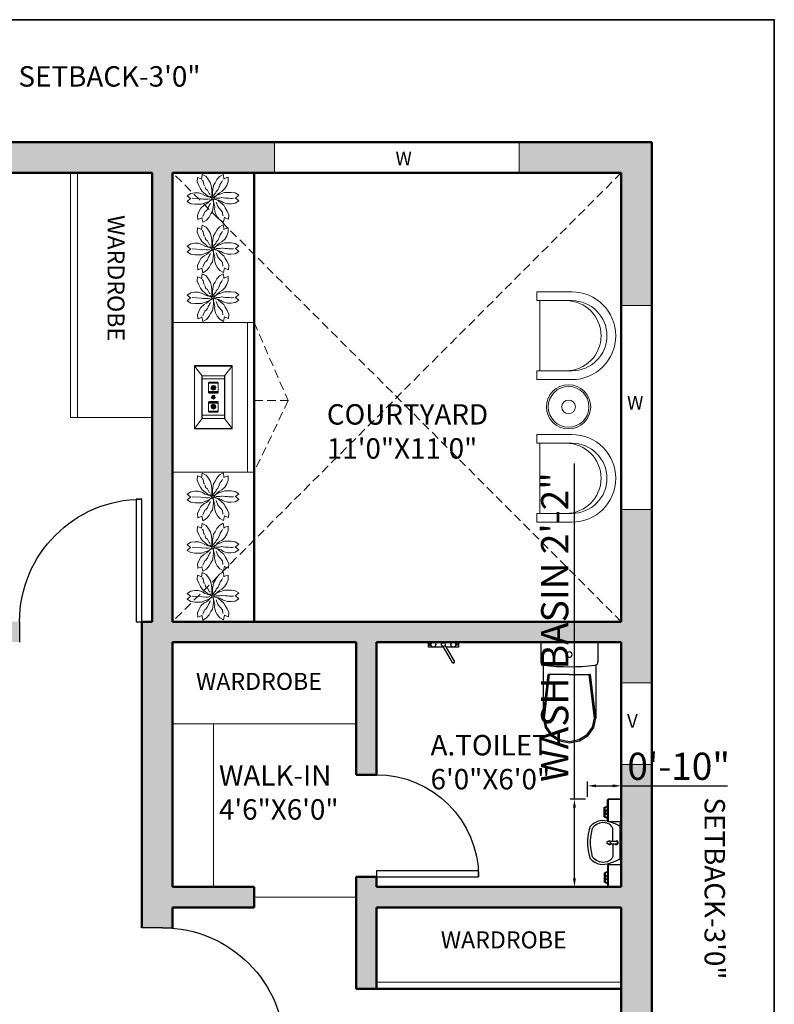
# Model space of a CAD drawing. Units: inches. Extents: x 3354 to 4308, y 1668 to 2317.
# Tile 11 of 11: x 4033 to 4255, y 2005 to 2294. Entities that reach past the tile are written whole.
import ezdxf

# ---------------------------------------------------------------- set-up
doc = ezdxf.new("R2010")
doc.units = ezdxf.units.IN
doc.linetypes.add('DASHED', pattern=[19.05, 12.7, -6.35])
for name, color, linetype, lineweight in [('A-ANNO-DIMS', 2, 'Continuous', 18), ('A-ANNO-TEXT', 7, 'Continuous', 18), ('A-AREA-IDEN', 3, 'Continuous', 18), ('A-DOOR', 3, 'Continuous', 25), ('A-FLOR-FIXT', 8, 'Continuous', 18), ('A-FLOR-OVHD', 8, 'DASHED', 18), ('A-FURN', 8, 'Continuous', 18), ('A-GLAZ', 4, 'Continuous', 18), ('A-WALL', 7, 'Continuous', 50), ('A-WALL-PATT', 8, 'Continuous', 13), ('C-PROP', 1, 'Continuous', 35), ('L-PLNT', 84, 'Continuous', 13)]:
    doc.layers.add(name, color=color, linetype=linetype, lineweight=lineweight)
doc.layers.add('SANTEH', color=7, linetype='Continuous')
doc.styles.get("Standard").update_dxf_attribs({"font": 'arial.ttf'})
doc.dimstyles.new('ISO-25', dxfattribs={"dimtxt": 8, "dimasz": 2.5, "dimexe": 1.25, "dimexo": 0.625, "dimtad": 1, "dimdec": 1, "dimlunit": 3, "dimtxsty": 'Standard', "dimcen": 2.5, "dimadec": 0, "dimazin": 0, "dimtfac": 1, "dimtdec": 1, "dimtmove": 0, "dimatfit": 3, "dimfxl": 1, "dimarcsym": 0})

# ---------------------------------------------------------------- blocks, each defined once
blk = doc.blocks.new('12PSTG07')
at = {"color": 0, "linetype": 'ByBlock'}
for p, q in [((0, 15), (-12, 15)), ((0, 12), (0, 15)), ((-12, 12), (0, 12)), ((-1, -12), (-1, 12)), ((-12, -12), (0, -12)), ((0, -12), (0, -15)), ((0, -15), (-12, -15))]:
    blk.add_line(p, q, dxfattribs=at)
for centre, radius in [((-12, 0), 15), ((-12, 0), 12), ((-10, 0), 12)]:
    blk.add_arc(centre, radius, 90, 270, dxfattribs=at)
blk = doc.blocks.new('*U3')
for p, q in [((0, 0), (0, -6)), ((36, 0), (36, -6))]:
    blk.add_line(p, q)
blk.add_lwpolyline([(0, 0), (0, 36), (1.75, 36), (1.75, 0)], close=True)
blk.add_arc((0, 0), 36, 0, 90)
blk = doc.blocks.new('ml')
for p, q in [((3455.3311, 1925.7742), (3455.3307, 1925.7627)), ((3455.3431, 1925.7698), (3455.3311, 1925.7742)), ((3455.3419, 1925.7691), (3455.3441, 1925.7817)), ((3455.3441, 1925.7817), (3455.3543, 1925.7763)), ((3455.3543, 1925.7763), (3455.3608, 1925.7679)), ((3455.3892, 1925.7768), (3455.3826, 1925.7684)), ((3455.3993, 1925.7823), (3455.3892, 1925.7768)), ((3455.4016, 1925.7697), (3455.3993, 1925.7823)), ((3455.4003, 1925.7704), (3455.4124, 1925.7747)), ((3455.4124, 1925.7747), (3455.4127, 1925.7632)), ((3455.3307, 1925.7627), (3455.3347, 1925.7528)), ((3455.3347, 1925.7528), (3455.3396, 1925.7443)), ((3455.3435, 1925.7672), (3455.3464, 1925.7643)), ((3455.3464, 1925.7643), (3455.3485, 1925.7554)), ((3455.3485, 1925.7554), (3455.3499, 1925.7524)), ((3455.3514, 1925.7499), (3455.3528, 1925.744)), ((3455.3608, 1925.7679), (3455.3657, 1925.7594)), ((3455.3657, 1925.7594), (3455.368, 1925.7482)), ((3455.368, 1925.7482), (3455.3679, 1925.7458)), ((3455.3688, 1925.7419), (3455.3679, 1925.7458)), ((3455.3721, 1925.7432), (3455.3738, 1925.7534)), ((3455.3738, 1925.7534), (3455.3777, 1925.76)), ((3455.3826, 1925.7684), (3455.3777, 1925.76)), ((3455.3855, 1925.743), (3455.3866, 1925.7454)), ((3455.3866, 1925.7454), (3455.3873, 1925.7469)), ((3455.3873, 1925.7469), (3455.3888, 1925.7494)), ((3455.3888, 1925.7494), (3455.3895, 1925.7504)), ((3455.3895, 1925.7504), (3455.3912, 1925.7564)), ((3455.3912, 1925.7564), (3455.3927, 1925.7588)), ((3455.3927, 1925.7588), (3455.3938, 1925.7598)), ((3455.3938, 1925.7598), (3455.3952, 1925.7623)), ((3455.3952, 1925.7623), (3455.3977, 1925.7658)), ((3455.4038, 1925.7449), (3455.3952, 1925.7373)), ((3455.4087, 1925.7534), (3455.4038, 1925.7449)), ((3455.4127, 1925.7632), (3455.4087, 1925.7534)), ((3455.304, 1925.7261), (3455.3138, 1925.7322)), ((3455.3138, 1925.7178), (3455.304, 1925.7261)), ((3455.3138, 1925.7193), (3455.304, 1925.711)), ((3455.3138, 1925.7322), (3455.3243, 1925.7337)), ((3455.317, 1925.7192), (3455.341, 1925.7177)), ((3455.3243, 1925.7337), (3455.3341, 1925.7337)), ((3455.3341, 1925.7337), (3455.345, 1925.73)), ((3455.3434, 1925.7376), (3455.3396, 1925.7443)), ((3455.3514, 1925.7311), (3455.3434, 1925.7376)), ((3455.345, 1925.73), (3455.3509, 1925.7263)), ((3455.3509, 1925.7263), (3455.3573, 1925.7241)), ((3455.3579, 1925.7256), (3455.3514, 1925.7311)), ((3455.3528, 1925.744), (3455.3579, 1925.7405)), ((3455.3573, 1925.7241), (3455.3659, 1925.7219)), ((3455.3579, 1925.7405), (3455.3622, 1925.7316)), ((3455.3656, 1925.7214), (3455.3579, 1925.7256)), ((3455.3622, 1925.7316), (3455.3639, 1925.7301)), ((3455.3639, 1925.7301), (3455.3647, 1925.7291)), ((3455.3643, 1925.7251), (3455.3672, 1925.7211)), ((3455.3707, 1925.7212), (3455.3656, 1925.7214)), ((3455.3659, 1925.7219), (3455.3697, 1925.7189)), ((3455.3697, 1925.7189), (3455.367, 1925.7145)), ((3455.3688, 1925.7216), (3455.3688, 1925.7419)), ((3455.3691, 1925.7345), (3455.3715, 1925.726)), ((3455.3707, 1925.7348), (3455.3721, 1925.7432)), ((3455.3708, 1925.726), (3455.3707, 1925.7348)), ((3455.3715, 1925.726), (3455.3707, 1925.7212)), ((3455.3733, 1925.7215), (3455.3708, 1925.726)), ((3455.3778, 1925.7232), (3455.3733, 1925.7215)), ((3455.3736, 1925.7261), (3455.3765, 1925.7301)), ((3455.3748, 1925.7194), (3455.3775, 1925.7238)), ((3455.3785, 1925.7164), (3455.3748, 1925.7194)), ((3455.3765, 1925.7301), (3455.3776, 1925.7316)), ((3455.3775, 1925.7238), (3455.385, 1925.7283)), ((3455.3776, 1925.7316), (3455.3794, 1925.7335)), ((3455.384, 1925.7296), (3455.3778, 1925.7232)), ((3455.3794, 1925.7335), (3455.3805, 1925.737)), ((3455.3798, 1925.7196), (3455.383, 1925.7196)), ((3455.3805, 1925.737), (3455.3826, 1925.739)), ((3455.3826, 1925.739), (3455.3848, 1925.7414)), ((3455.383, 1925.7196), (3455.3905, 1925.7196)), ((3455.3891, 1925.734), (3455.384, 1925.7296)), ((3455.3848, 1925.7414), (3455.3855, 1925.743)), ((3455.385, 1925.7283), (3455.393, 1925.7312)), ((3455.3952, 1925.7373), (3455.3891, 1925.734)), ((3455.3905, 1925.7196), (3455.3945, 1925.7211)), ((3455.393, 1925.7312), (3455.4026, 1925.7349)), ((3455.3945, 1925.7211), (3455.397, 1925.7211)), ((3455.3995, 1925.7206), (3455.4045, 1925.7196)), ((3455.4026, 1925.7349), (3455.4103, 1925.7348)), ((3455.4045, 1925.7196), (3455.4103, 1925.7196)), ((3455.4201, 1925.7348), (3455.4103, 1925.7348)), ((3455.4103, 1925.7196), (3455.4139, 1925.7192)), ((3455.4139, 1925.7192), (3455.4189, 1925.7187)), ((3455.4189, 1925.7187), (3455.4225, 1925.7187)), ((3455.4306, 1925.7333), (3455.4201, 1925.7348)), ((3455.4225, 1925.7187), (3455.426, 1925.7192)), ((3455.4404, 1925.7273), (3455.4306, 1925.7333)), ((3455.4306, 1925.719), (3455.4404, 1925.7273)), ((3455.4306, 1925.7205), (3455.4404, 1925.7122)), ((3455.304, 1925.711), (3455.3138, 1925.705)), ((3455.3138, 1925.705), (3455.3243, 1925.7035)), ((3455.3243, 1925.7035), (3455.3341, 1925.7035)), ((3455.3418, 1925.7034), (3455.3341, 1925.7035)), ((3455.3357, 1925.6849), (3455.3406, 1925.6934)), ((3455.3406, 1925.6934), (3455.3492, 1925.701)), ((3455.341, 1925.7177), (3455.3453, 1925.7167)), ((3455.3514, 1925.7071), (3455.3418, 1925.7034)), ((3455.3453, 1925.7167), (3455.3489, 1925.7172)), ((3455.3489, 1925.7172), (3455.3543, 1925.7167)), ((3455.3492, 1925.701), (3455.3553, 1925.7043)), ((3455.3595, 1925.71), (3455.3514, 1925.7071)), ((3455.3543, 1925.7167), (3455.3597, 1925.7167)), ((3455.3553, 1925.7043), (3455.3605, 1925.7088)), ((3455.3582, 1925.6924), (3455.3597, 1925.6949)), ((3455.367, 1925.7145), (3455.3595, 1925.71)), ((3455.3597, 1925.7167), (3455.3636, 1925.7177)), ((3455.3597, 1925.6949), (3455.3608, 1925.6974)), ((3455.3605, 1925.7088), (3455.3667, 1925.7151)), ((3455.3608, 1925.6974), (3455.3618, 1925.6993)), ((3455.3618, 1925.6993), (3455.3632, 1925.7023)), ((3455.3632, 1925.7023), (3455.3647, 1925.7048)), ((3455.3647, 1925.7048), (3455.3661, 1925.7067)), ((3455.3667, 1925.7151), (3455.3712, 1925.7168)), ((3455.3723, 1925.6951), (3455.3706, 1925.6849)), ((3455.3712, 1925.7168), (3455.3736, 1925.7123)), ((3455.3738, 1925.7035), (3455.3723, 1925.6951)), ((3455.373, 1925.7123), (3455.3737, 1925.7171)), ((3455.3753, 1925.7038), (3455.373, 1925.7123)), ((3455.3736, 1925.7123), (3455.3738, 1925.7035)), ((3455.3737, 1925.7171), (3455.3789, 1925.7169)), ((3455.3767, 1925.6971), (3455.3753, 1925.7038)), ((3455.3764, 1925.6901), (3455.3767, 1925.6971)), ((3455.3871, 1925.7142), (3455.3785, 1925.7164)), ((3455.3789, 1925.7169), (3455.3865, 1925.7127)), ((3455.3804, 1925.7089), (3455.385, 1925.6972)), ((3455.385, 1925.6972), (3455.3976, 1925.683)), ((3455.3865, 1925.7127), (3455.3931, 1925.7072)), ((3455.3935, 1925.712), (3455.3871, 1925.7142)), ((3455.3931, 1925.7072), (3455.4011, 1925.7007)), ((3455.3994, 1925.7083), (3455.3935, 1925.712)), ((3455.4103, 1925.7046), (3455.3994, 1925.7083)), ((3455.4011, 1925.7007), (3455.4048, 1925.694)), ((3455.4097, 1925.6855), (3455.4048, 1925.694)), ((3455.4201, 1925.7046), (3455.4103, 1925.7046)), ((3455.4306, 1925.7061), (3455.4201, 1925.7046)), ((3455.4404, 1925.7122), (3455.4306, 1925.7061)), ((3455.3317, 1925.6751), (3455.3357, 1925.6849)), ((3455.3321, 1925.6636), (3455.3317, 1925.6751)), ((3455.3441, 1925.6679), (3455.3321, 1925.6636)), ((3455.3429, 1925.6686), (3455.3451, 1925.656)), ((3455.3457, 1925.6716), (3455.3504, 1925.6835)), ((3455.3504, 1925.6835), (3455.3532, 1925.6849)), ((3455.3532, 1925.6849), (3455.355, 1925.6874)), ((3455.355, 1925.6874), (3455.3575, 1925.6904)), ((3455.3553, 1925.6615), (3455.3618, 1925.6699)), ((3455.3575, 1925.6904), (3455.3582, 1925.6924)), ((3455.3618, 1925.6699), (3455.3667, 1925.6783)), ((3455.3706, 1925.6849), (3455.3667, 1925.6783)), ((3455.3787, 1925.6789), (3455.3764, 1925.6901)), ((3455.3836, 1925.6704), (3455.3787, 1925.6789)), ((3455.3902, 1925.662), (3455.3836, 1925.6704)), ((3455.3976, 1925.683), (3455.3985, 1925.6734)), ((3455.4026, 1925.6692), (3455.4003, 1925.6566)), ((3455.4013, 1925.6685), (3455.4134, 1925.6641)), ((3455.4137, 1925.6756), (3455.4097, 1925.6855)), ((3455.4134, 1925.6641), (3455.4137, 1925.6756)), ((3455.3451, 1925.656), (3455.3553, 1925.6615)), ((3455.4003, 1925.6566), (3455.3902, 1925.662))]:
    blk.add_line(p, q)
blk = doc.blocks.new('12PLMP48')
for p, q in [((-4.94, 8.22), (-5, 8.31)), ((-5, 8.31), (5, 8.31)), ((-5, -8.31), (-5, 8.31)), ((-2.96, 5.62), (-4.94, 8.22)), ((4.94, 8.22), (-4.94, 8.22)), ((-4.94, 8.22), (-4.94, -8.22)), ((2.96, 5.62), (4.94, 8.22)), ((5, 8.31), (4.94, 8.22)), ((4.94, 8.22), (4.94, -8.22)), ((5, 8.31), (5, -8.31)), ((-2.94, 5.59), (-3, 5.62)), ((-3, 5.62), (3, 5.62)), ((-3, -5.63), (-3, 5.62)), ((2.94, 5.59), (-2.94, 5.59)), ((-2.94, 5.59), (-2.94, -5.59)), ((3, 5.62), (2.94, 5.59)), ((2.94, -5.59), (2.94, 5.59)), ((3, -5.63), (3, 5.62)), ((2.94, 4.81), (-2.94, 4.81)), ((-1.13, 3.94), (-1.25, 3.81)), ((-1.13, 3.84), (-1.25, 3.72)), ((-1.25, 3.81), (-1.25, 1.22)), ((-1.25, 3.72), (1.25, 3.72)), ((1.13, 3.94), (-1.13, 3.94)), ((-1.13, 3.84), (-1.13, 3.94)), ((1.13, 3.84), (-1.13, 3.84)), ((-0.62, 2.61), (-0.4, 2.98)), ((0, 2.5), (-0.62, 2.61)), ((-0.54, 2.19), (-0.62, 2.61)), ((-0.32, 2.88), (-0.49, 2.59)), ((-0.43, 2.58), (-0.28, 2.83)), ((0, 3.12), (-0.4, 2.98)), ((-0.4, 2.98), (-0.32, 2.88)), ((0, 3), (-0.32, 2.88)), ((-0.32, 2.88), (-0.32, 2.88)), ((-0.32, 2.88), (-0.28, 2.83)), ((-0.28, 2.83), (0, 2.94)), ((-0.28, 2.83), (0, 2.5)), ((-0.08, 2.6), (-0.12, 2.52)), ((0, 2.62), (-0.08, 2.6)), ((0, 2.5), (0, 3.12)), ((0, 3.12), (0.4, 2.98)), ((0.32, 2.88), (0, 3)), ((0, 2.94), (0.28, 2.83)), ((0, 2.5), (0.32, 2.88)), ((0.08, 2.6), (0, 2.62)), ((0.62, 2.61), (0, 2.5)), ((0.12, 2.52), (0.08, 2.6)), ((0.28, 2.83), (0.43, 2.58)), ((0.32, 2.88), (0.4, 2.98)), ((0.49, 2.59), (0.32, 2.88)), ((0.32, 2.88), (0.32, 2.88)), ((0.4, 2.98), (0.62, 2.61)), ((0.54, 2.19), (0.62, 2.61)), ((1.25, 3.81), (1.13, 3.94)), ((1.13, 3.84), (1.13, 3.94)), ((1.25, 3.72), (1.13, 3.84)), ((1.25, 1.22), (1.25, 3.81)), ((-1.13, 1.41), (-1.25, 1.53)), ((-1.25, 1.53), (1.25, 1.53)), ((-1.13, 1.25), (-1.25, 1.37)), ((-1.25, 1.22), (-1.13, 1.09)), ((1.13, 1.41), (-1.13, 1.41)), ((-1.13, 1.41), (-1.13, 1.09)), ((-1.13, 1.25), (1.13, 1.25)), ((-1.13, 1.09), (1.13, 1.09)), ((-0.38, 2.28), (-0.54, 2.19)), ((-0.54, 2.19), (-0.21, 1.91)), ((-0.49, 2.59), (-0.43, 2.25)), ((-0.49, -0.09), (-0.43, 0.25)), ((-0.38, 2.28), (-0.43, 2.58)), ((-0.43, 2.25), (-0.17, 2.03)), ((-0.43, 0.25), (-0.17, 0.47)), ((0, 2.5), (-0.38, 2.28)), ((-0.15, 2.09), (-0.38, 2.28)), ((-0.22, 0.12), (-0.25, -0.04)), ((-0.09, 0.23), (-0.22, 0.12)), ((-0.21, 1.91), (0, 2.5)), ((0.21, 1.91), (-0.21, 1.91)), ((-0.17, 2.03), (0.17, 2.03)), ((0.17, 0.47), (-0.17, 0.47)), ((0.15, 2.09), (-0.15, 2.09)), ((-0.12, 2.52), (-0.11, 2.44)), ((-0.12, -0.12), (-0.12, 0.12)), ((-0.12, 0.12), (0.12, 0.12)), ((-0.11, 2.44), (-0.04, 2.38)), ((-0.09, 0.23), (0.09, 0.23)), ((-0.04, 2.38), (0.04, 2.38)), ((0.54, 2.19), (0, 2.5)), ((0, 2.5), (0.21, 1.91)), ((0.04, 2.38), (0.11, 2.44)), ((0.22, 0.12), (0.09, 0.23)), ((0.11, 2.44), (0.12, 2.52)), ((0.12, 0.12), (0.12, -0.12)), ((0.38, 2.28), (0.15, 2.09)), ((0.17, 2.03), (0.43, 2.25)), ((0.43, 0.25), (0.17, 0.47)), ((0.21, 1.91), (0.54, 2.19)), ((0.25, -0.04), (0.22, 0.12)), ((0.43, 2.58), (0.38, 2.28)), ((0.43, 2.25), (0.49, 2.59)), ((0.43, 0.25), (0.49, -0.09)), ((1.25, 1.53), (1.13, 1.41)), ((1.13, 1.09), (1.13, 1.41)), ((1.13, 1.25), (1.25, 1.37)), ((1.13, 1.09), (1.25, 1.22)), ((-1.25, -1.22), (-1.13, -1.09)), ((-1.25, -1.22), (-1.25, -3.81)), ((-1.13, -1.25), (-1.25, -1.38)), ((-1.13, -1.41), (-1.25, -1.53)), ((-1.25, -1.53), (1.25, -1.53)), ((-1.13, -1.41), (-1.13, -1.09)), ((-1.13, -1.09), (1.13, -1.09)), ((1.13, -1.25), (-1.13, -1.25)), ((1.13, -1.41), (-1.13, -1.41)), ((-0.54, -2.19), (-0.62, -2.61)), ((0, -2.5), (-0.62, -2.61)), ((-0.21, -1.91), (-0.54, -2.19)), ((-0.54, -2.19), (0, -2.5)), ((-0.32, -0.38), (-0.49, -0.09)), ((-0.49, -2.59), (-0.43, -2.25)), ((-0.32, -2.88), (-0.49, -2.59)), ((-0.43, -2.25), (-0.17, -2.03)), ((-0.43, -2.58), (-0.38, -2.28)), ((-0.28, -2.84), (-0.43, -2.58)), ((-0.38, -2.28), (-0.15, -2.09)), ((-0.32, -0.38), (0, -0.5)), ((-0.16, -0.19), (-0.25, -0.04)), ((0.21, -1.91), (-0.21, -1.91)), ((0, -2.5), (-0.21, -1.91)), ((-0.17, -2.03), (0.17, -2.03)), ((0, -0.25), (-0.16, -0.19)), ((-0.15, -2.09), (0.15, -2.09)), ((0.12, -0.12), (-0.12, -0.12)), ((-0.11, -2.44), (-0.12, -2.52)), ((-0.12, -2.52), (-0.08, -2.6)), ((-0.04, -2.38), (-0.11, -2.44)), ((-0.08, -2.6), (0, -2.5)), ((0.04, -2.38), (-0.04, -2.38)), ((0.16, -0.19), (0, -0.25)), ((0.32, -0.38), (0, -0.5)), ((0, -2.5), (0.21, -1.91)), ((0.11, -2.44), (0, -2.5)), ((0, -3.13), (0, -2.5)), ((0, -2.5), (0.4, -2.98)), ((0.62, -2.61), (0, -2.5)), ((0.11, -2.44), (0.04, -2.38)), ((0.08, -2.6), (0.12, -2.52)), ((0.38, -2.28), (0.11, -2.44)), ((0.12, -2.52), (0.11, -2.44)), ((0.15, -2.09), (0.38, -2.28)), ((0.16, -0.19), (0.25, -0.04)), ((0.17, -2.03), (0.43, -2.25)), ((0.21, -1.91), (0.54, -2.19)), ((0.43, -2.58), (0.28, -2.84)), ((0.32, -0.38), (0.49, -0.09)), ((0.49, -2.59), (0.32, -2.88)), ((0.54, -2.19), (0.38, -2.28)), ((0.38, -2.28), (0.43, -2.58)), ((0.43, -2.25), (0.49, -2.59)), ((0.62, -2.61), (0.54, -2.19)), ((1.13, -1.41), (1.13, -1.09)), ((1.13, -1.09), (1.25, -1.22)), ((1.25, -1.38), (1.13, -1.25)), ((1.25, -1.53), (1.13, -1.41)), ((1.25, -3.81), (1.25, -1.22)), ((2.94, -4.69), (-2.94, -4.69)), ((-1.13, -3.84), (-1.25, -3.72)), ((-1.25, -3.72), (1.25, -3.72)), ((-1.25, -3.81), (-1.13, -3.94)), ((-1.13, -3.94), (-1.13, -3.84)), ((1.13, -3.84), (-1.13, -3.84)), ((-1.13, -3.94), (1.13, -3.94)), ((-0.62, -2.61), (-0.4, -2.98)), ((-0.4, -2.98), (-0.32, -2.88)), ((-0.4, -2.98), (0, -3.13)), ((-0.32, -2.88), (-0.28, -2.84)), ((0, -3), (-0.32, -2.88)), ((-0.28, -2.84), (-0.08, -2.6)), ((0, -2.94), (-0.28, -2.84)), ((-0.08, -2.6), (0, -2.63)), ((0, -2.63), (0.08, -2.6)), ((0.28, -2.84), (0, -2.94)), ((0.32, -2.88), (0, -3)), ((0, -3.13), (0.4, -2.98)), ((0.4, -2.98), (0.62, -2.61)), ((1.25, -3.72), (1.13, -3.84)), ((1.13, -3.94), (1.25, -3.81)), ((1.13, -3.94), (1.13, -3.84)), ((-4.94, -8.22), (-2.96, -5.63)), ((-2.94, -5.59), (-3, -5.63)), ((-3, -5.63), (3, -5.63)), ((-2.94, -5.59), (2.94, -5.59)), ((3, -5.63), (2.94, -5.59)), ((2.96, -5.63), (4.94, -8.22)), ((-4.94, -8.22), (-5, -8.31)), ((5, -8.31), (-5, -8.31)), ((4.94, -8.22), (-4.94, -8.22)), ((4.94, -8.22), (5, -8.31))]:
    blk.add_line(p, q)
blk = doc.blocks.new('*U2')
for p, q in [((0, 0), (0, -6)), ((30, 0), (30, -6))]:
    blk.add_line(p, q)
blk.add_lwpolyline([(0, 0), (0, 30), (1.75, 30), (1.75, 0)], close=True)
blk.add_arc((0, 0), 30, 0, 90)
blk = doc.blocks.new('WC 2 Symb_109')
at = {"layer": 'SANTEH'}
for p, q in [((0, 0), (0, 380)), ((0, 380), (132.4, 380)), ((153.6, 364.9), (506.8, 364.9)), ((506.3, 364.9), (215.7, 330.9)), ((506.3, 356), (215.7, 322)), ((215.7, 190), (215.7, 330.9)), ((215.7, 190), (215.7, 49.1)), ((153.8, 15.1), (506.8, 15.1)), ((506.3, 24), (215.7, 58)), ((506.3, 15.1), (215.7, 49.1)), ((0, 0), (132.4, 0))]:
    blk.add_line(p, q, dxfattribs=at)
for points in [[(154.6, 360.1), (153.9, 364.1), (152.3, 367.9), (150.2, 371.3), (147.4, 374.3), (144.1, 376.7), (140.5, 378.5), (136.5, 379.6), (132.4, 380)], [(154.6, 19.7), (158.6, 62.1), (161.4, 104.7), (163.1, 147.3), (163.7, 189.9), (163.1, 232.5), (161.4, 275.1), (158.6, 317.7), (154.6, 360.1)], [(506.3, 24), (565.5, 36.6), (615.7, 72.6), (649.2, 126.5), (661, 190), (649.2, 253.5), (615.7, 307.4), (565.5, 343.4), (506.3, 356)], [(506.8, 15.1), (569.2, 28.4), (622.2, 66.3), (657.6, 123.1), (670, 190), (657.6, 256.9), (622.2, 313.7), (569.2, 351.6), (506.8, 364.9)], [(132.4, 0), (136.5, 0.4), (140.4, 1.5), (144.1, 3.2), (147.3, 5.6), (150.1, 8.6), (152.3, 12), (153.8, 15.7), (154.6, 19.7)]]:
    blk.add_lwpolyline(points, dxfattribs=at)
blk.add_lwpolyline([(83.6, 208.5), (70.4, 203.1), (64.9, 190), (70.4, 176.9), (83.6, 171.5), (96.8, 176.9), (102.2, 190), (96.8, 203.1)], close=True, dxfattribs=at)
blk = doc.blocks.new('Faucet - kit sink top')
at = {"layer": 'SANTEH'}
for p, q in [((-5.5, -0.75), (-5.5, -1.25)), ((-4.94278, -0.75), (-5.5, -0.75)), ((-5.5, -1.25), (-4.94278, -1.25)), ((-0.14775, -1.7441), (3.56698, -8.1782)), ((4.43301, -7.6782), (0.71828, -1.2441)), ((4.94278, -0.75), (5.5, -0.75)), ((5.5, -1.25), (4.94278, -1.25)), ((5.5, -0.75), (5.5, -1.25))]:
    blk.add_line(p, q, dxfattribs=at)
blk.add_lwpolyline([(-0.00587, -2), (-6, -2), (-6, 0), (6, 0), (6, -2), (1.15195, -2)], dxfattribs=at)
for centre, radius in [((-4, -1), 1), ((4, -1), 1), ((0, -1), 0.75)]:
    blk.add_circle(centre, radius, dxfattribs=at)
blk.add_arc((4, -7.9282), 0.5, 210, 30, dxfattribs=at)
blk = doc.blocks.new('s_42')
at = {"layer": 'SANTEH'}
for p, q in [((-189.37677, -27.989292), (-189.37677, 0)), ((-189.37677, -0.040064), (-96.48379, -0.039864)), ((-140.166604, -27.989292), (-140.166604, 0)), ((-140.147078, -26.702214), (-140.147078, 0)), ((-140.057622, -26.58844), (-140.057622, 0)), ((-138.936126, -30.19495), (-135.551368, -19.131184)), ((-135.551368, -19.131184), (-131.511318, -9.749604)), ((-85.572468, 0), (-132.584582, 0)), ((-131.511318, -9.749604), (-128.12637, -3.244686)), ((-127.328526, -20.699978), (-131.143938, -24.38097)), ((-130.030858, -1.697254), (-50.75196, -1.697254)), ((-130.030858, -3.067398), (-130.030858, -1.697254)), ((-50.75196, -3.067398), (-130.030858, -3.067398)), ((-128.12637, -3.244686), (-128.022848, -3.067398)), ((-124.131834, -18.954276), (-127.328526, -20.699978)), ((-127.223836, -1.697254), (-126.706826, -0.811004)), ((-126.706826, -0.811004), (-116.815434, -0.805282)), ((-58.157026, -0.811004), (-126.706826, -0.811004)), ((-122.791396, -18.51263), (-124.131834, -18.954276)), ((-95.518552, -18.51263), (-122.791396, -18.51263)), ((-116.815434, -0.805282), (-106.126558, -0.797272)), ((-106.126558, -0.797272), (-78.706634, -0.797272)), ((-96.851574, -11.067582), (-96.636926, -9.463214)), ((-96.440422, -12.63256), (-96.851574, -11.067582)), ((-96.636926, -9.463214), (-95.829498, -8.063602)), ((-96.48379, -0.797272), (-96.48379, 0)), ((-96.48379, -0.811004), (-96.48379, -0.805282)), ((-95.518552, -13.850784), (-96.440422, -12.63256)), ((-95.829498, -8.063602), (-94.551766, -7.081986)), ((-95.518552, -10.585022), (-94.786322, -9.3688)), ((-95.518552, -29.093742), (-95.518552, -10.400868)), ((-95.518552, -21.430016), (-94.79922, -22.660446)), ((-94.786322, -9.3688), (-93.811714, -8.63905)), ((-94.551766, -7.081986), (-92.998444, -6.667804)), ((-93.811714, -8.63905), (-92.71835, -8.395862)), ((-92.998444, -6.667804), (-91.406046, -6.883908)), ((-92.71835, -8.395862), (-91.630088, -8.63905)), ((-91.630088, -8.63905), (-90.671098, -9.3688)), ((-91.406046, -6.883908), (-90.016996, -7.697582)), ((-90.683996, -22.660446), (-89.96464, -21.430016)), ((-90.671098, -9.3688), (-89.96464, -10.585022)), ((-90.016996, -7.697582), (-89.04277, -8.984948)), ((-89.96464, -10.585022), (-89.96464, -10.400868)), ((-89.96464, -10.585022), (-89.96464, -21.430016)), ((-89.96464, -18.51263), (-61.574208, -18.51263)), ((-89.96464, -21.430016), (-89.96464, -29.093742)), ((-89.04277, -8.984948), (-88.63164, -10.549926)), ((-88.329112, -0.797272), (-88.329112, 0)), ((-88.329112, -0.039864), (-46.888864, -0.039864)), ((-88.329112, -0.811004), (-88.329112, -0.805282)), ((-78.706634, -0.797272), (-68.033802, -0.805282)), ((-68.033802, -0.805282), (-58.157026, -0.811004)), ((-61.574208, -18.51263), (-60.280262, -18.954276)), ((-60.280262, -18.954276), (-57.19453, -20.699978)), ((-58.157026, -0.811004), (-57.638274, -1.697254)), ((-57.19453, -20.699978), (-53.511536, -24.38097)), ((-56.83614, -3.067398), (-56.732236, -3.244686)), ((-56.732236, -3.244686), (-53.334772, -9.749604)), ((-53.334772, -9.749604), (-49.279486, -19.131184)), ((-50.75196, -1.697254), (-50.75196, -3.067398)), ((-49.279486, -19.131184), (-46.888864, -26.916218)), ((-46.888864, -0.039386), (2.321292, -0.039386)), ((-46.888864, -28.821086), (-46.888864, -0.039386)), ((-44.416998, -0.039386), (-44.416998, 0)), ((0, -0.039386), (0, 0)), ((2.321292, -0.039386), (2.321292, -28.821086)), ((2.321292, -0.068282), (2.430274, -0.068282)), ((2.340818, -0.101662), (2.321292, -0.101662)), ((2.340818, -27.534104), (2.340818, -0.101662)), ((2.430274, -0.068282), (2.430274, -27.42033)), ((-188.006842, -29.359436), (-189.37677, -27.989292)), ((-189.37677, -27.989292), (-140.166604, -27.989292)), ((-141.536724, -29.359436), (-188.006842, -29.359436)), ((-187.548434, -29.359436), (-187.328136, -29.579926)), ((-187.328136, -29.579926), (-142.240822, -29.579926)), ((-187.25723, -29.579926), (-187.205088, -29.631996)), ((-182.532416, -29.579926), (-178.656064, -36.429406)), ((-178.656064, -36.429406), (-182.502924, -29.631996)), ((-180.635154, -29.579926), (-178.656064, -34.455776)), ((-178.656064, -34.455776), (-166.725194, -34.455776)), ((-178.656064, -34.455776), (-171.805464, -34.455776)), ((-178.656064, -36.429406), (-166.725194, -36.429406)), ((-171.805464, -34.455776), (-174.56504, -29.579926)), ((-170.688474, -34.455776), (-172.667586, -29.579926)), ((-166.725194, -34.455776), (-170.688474, -34.455776)), ((-164.799606, -29.579926), (-166.725194, -34.455776)), ((-166.725194, -36.429406), (-162.79491, -29.579926)), ((-166.725194, -34.455776), (-164.82011, -29.631996)), ((-166.725194, -36.429406), (-158.757626, -36.429406)), ((-165.592776, -34.455776), (-158.757626, -34.455776)), ((-158.757626, -34.455776), (-156.83223, -29.579926)), ((-158.757626, -36.429406), (-154.827534, -29.579926)), ((-142.41153, -29.631996), (-142.359386, -29.579926)), ((-142.240822, -29.579926), (-142.020498, -29.359436)), ((-140.166604, -27.989292), (-141.536724, -29.359436)), ((-140.35567, -41.746616), (-138.936126, -30.19495)), ((-138.930856, -50.152302), (-140.35567, -41.746616)), ((-140.166604, -26.702214), (-140.147078, -26.702214)), ((-140.147078, -26.58844), (-140.057622, -26.58844)), ((-134.340632, -30.628204), (-135.681258, -40.073108)), ((-135.681258, -40.073108), (-134.461318, -47.948552)), ((-131.143938, -24.38097), (-134.340632, -30.628204)), ((-96.435748, -23.943806), (-96.778524, -27.132702)), ((-96.778524, -27.132702), (-96.55801, -25.081348)), ((-96.778524, -27.132702), (-95.518552, -28.688336)), ((-95.518552, -23.207092), (-96.435748, -23.943806)), ((-94.79922, -22.660446), (-93.832432, -23.39878)), ((-93.832432, -23.39878), (-92.741596, -23.644924)), ((-92.741596, -23.644924), (-91.650784, -23.39878)), ((-91.650784, -23.39878), (-90.683996, -22.660446)), ((-88.70586, -24.768066), (-89.96464, -23.213768)), ((-89.96464, -28.692626), (-89.048636, -27.956868)), ((-89.048636, -27.956868), (-88.70586, -24.768066)), ((-53.511536, -24.38097), (-50.425778, -30.628204)), ((-50.425778, -30.628204), (-49.131642, -40.073108)), ((-49.131642, -40.073108), (-50.356828, -47.948552)), ((-46.888864, -28.821086), (-45.518946, -30.191326)), ((2.321292, -28.821086), (-46.888864, -28.821086)), ((-46.044528, -29.665566), (-45.882034, -30.19495)), ((-45.882034, -30.19495), (-44.457232, -41.746616)), ((-44.457232, -41.746616), (-45.882034, -50.152302)), ((-45.518946, -30.191326), (0.951172, -30.191326)), ((-45.06055, -30.191326), (-44.84024, -30.41172)), ((-44.84024, -30.41172), (0.247074, -30.41172)), ((-44.769334, -30.41172), (-44.717192, -30.463886)), ((-40.044534, -30.41172), (-36.16817, -37.2612)), ((-36.16817, -37.2612), (-40.01504, -30.463886)), ((-38.14727, -30.41172), (-36.16817, -35.28757)), ((-36.16817, -35.28757), (-24.23731, -35.28757)), ((-36.16817, -35.28757), (-29.31758, -35.28757)), ((-36.16817, -37.2612), (-24.23731, -37.2612)), ((-29.31758, -35.28757), (-32.077144, -30.41172)), ((-28.20059, -35.28757), (-30.17969, -30.41172)), ((-24.23731, -35.28757), (-28.20059, -35.28757)), ((-22.311722, -30.41172), (-24.23731, -35.28757)), ((-24.23731, -37.2612), (-20.307028, -30.41172)), ((-24.23731, -35.28757), (-22.332226, -30.463886)), ((-24.23731, -37.2612), (-16.26973, -37.2612)), ((-23.104882, -35.28757), (-16.26973, -35.28757)), ((-16.26973, -35.28757), (-14.344334, -30.41172)), ((-16.26973, -37.2612), (-12.33965, -30.41172)), ((0.076366, -30.463886), (0.12852, -30.41172)), ((0.247074, -30.41172), (0.467384, -30.191326)), ((0.951172, -30.191326), (2.321292, -28.821086)), ((2.321292, -27.534104), (2.340818, -27.534104)), ((2.430274, -27.42033), (2.340818, -27.42033)), ((-135.533392, -57.61509), (-138.930856, -50.152302)), ((-131.47813, -63.603402), (-135.533392, -57.61509)), ((-134.461318, -47.948552), (-131.552732, -54.304694)), ((-131.552732, -54.304694), (-128.081046, -59.00898)), ((-128.081046, -67.586136), (-131.47813, -63.603402)), ((-128.081046, -59.00898), (-125.17246, -61.928844)), ((-125.17246, -61.928844), (-123.952542, -62.931538)), ((-123.952542, -62.931538), (-108.56992, -65.8782)), ((-76.452744, -65.8782), (-60.910546, -62.931538)), ((-59.685552, -61.928844), (-60.910546, -62.931538)), ((-56.764446, -59.00898), (-59.685552, -61.928844)), ((-53.277932, -54.304694), (-56.764446, -59.00898)), ((-53.334772, -63.603402), (-56.732236, -67.586136)), ((-49.279486, -57.61509), (-53.334772, -63.603402)), ((-50.356828, -47.948552), (-53.277932, -54.304694)), ((-45.882034, -50.152302), (-49.279486, -57.61509)), ((-126.655852, -69.031716), (-128.081046, -67.586136)), ((-110.586536, -72.015858), (-126.655852, -69.031716)), ((-98.152148, -73.507882), (-110.586536, -72.015858)), ((-108.56992, -65.8782), (-97.428332, -67.351436)), ((-86.902724, -73.507882), (-98.152148, -73.507882)), ((-97.428332, -67.351436), (-87.673818, -67.351532)), ((-87.673818, -67.351532), (-76.452744, -65.8782)), ((-74.387896, -72.015858), (-86.902724, -73.507882)), ((-58.157026, -69.031716), (-74.387896, -72.015858)), ((-56.732236, -67.586136), (-58.157026, -69.031716))]:
    blk.add_line(p, q, dxfattribs=at)
blk.add_arc((-92.741596, -28.241466), 2.904799, 197.061787614, 342.938212386, dxfattribs=at)
blk = doc.blocks.new('*D96')
at = {"layer": 'A-ANNO-DIMS', "color": 0, "lineweight": -2, "transparency": 16777216}
for p, q in [((4196.54, 2065.16), (4196.54, 2163.78)), ((4199.8, 2065.16), (4195.29, 2065.16)), ((4196.54, 2041.8), (4196.54, 2062.66)), ((4199.8, 2039.3), (4195.29, 2039.3))]:
    blk.add_line(p, q, dxfattribs=at)
at = {"layer": 'A-ANNO-DIMS', "color": 0, "transparency": 16777216}
for points in [[(4196.13, 2062.66), (4196.96, 2062.66), (4196.54, 2065.16)], [(4196.13, 2041.8), (4196.96, 2041.8), (4196.54, 2039.3)]]:
    blk.add_solid(points, dxfattribs=at)
at = {"layer": 'Defpoints', "color": 0, "transparency": 16777216}
for p in [(4196.54, 2065.16), (4200.42, 2065.16), (4200.42, 2039.3)]:
    blk.add_point(p, dxfattribs=at)
at = {"layer": 'A-ANNO-DIMS', "color": 0, "transparency": 16777216, "insert": (4191.78, 2115.72), "char_height": 8, "attachment_point": 5, "rotation": 90}
blk.add_mtext('WASH BASIN 2\'-2"', dxfattribs=at)
blk = doc.blocks.new('*D97')
at = {"layer": 'A-ANNO-DIMS', "color": 0, "lineweight": -2, "transparency": 16777216}
for p, q in [((4200.42, 2065.78), (4200.42, 2070.29)), ((4210.33, 2065.78), (4210.33, 2070.29)), ((4202.92, 2069.04), (4207.83, 2069.04)), ((4210.33, 2069.04), (4241.57, 2069.04))]:
    blk.add_line(p, q, dxfattribs=at)
at = {"layer": 'A-ANNO-DIMS', "color": 0, "transparency": 16777216}
for points in [[(4202.92, 2069.45), (4202.92, 2068.62), (4200.42, 2069.04)], [(4207.83, 2069.45), (4207.83, 2068.62), (4210.33, 2069.04)]]:
    blk.add_solid(points, dxfattribs=at)
at = {"layer": 'Defpoints', "color": 0, "transparency": 16777216}
for p in [(4210.33, 2069.04), (4200.42, 2065.16), (4210.33, 2065.16)]:
    blk.add_point(p, dxfattribs=at)
at = {"layer": 'A-ANNO-DIMS', "color": 0, "transparency": 16777216, "insert": (4227.2, 2073.75), "char_height": 8, "attachment_point": 5}
blk.add_mtext('0\'-10"', dxfattribs=at)

msp = doc.modelspace()

# ---------------------------------------------------------------- hatches: boundary and pattern name
at = {"layer": 'A-WALL-PATT', "transparency": 33554687}
h = msp.add_hatch(color=256, dxfattribs=at)
h.dxf.hatch_style = 1
h.paths.add_polyline_path([(4078.33, 1991.3), (4069.33, 1991.3), (4069.33, 1961.3), (4063.33, 1961.3), (4063.33, 1955.3), (4069.33, 1955.3), (4069.33, 1808.3), (4078.33, 1808.3), (4078.33, 1829.3), (4108.33, 1829.3), (4108.33, 1838.3), (4078.33, 1838.3)])
h.paths.add_polyline_path([(4219.33, 1850.3), (4210.33, 1850.3), (4210.33, 1838.3), (4180.33, 1838.3), (4180.33, 1829.3), (4219.33, 1829.3)])
h.paths.add_polyline_path([(4219.33, 2075.3), (4210.33, 2075.3), (4210.33, 2039.3), (4206.56, 2039.3), (4138.33, 2039.3), (4138.33, 2042.3), (4132.33, 2042.3), (4132.33, 2009.3), (4138.33, 2009.3), (4138.33, 2033.3), (4210.33, 2033.3), (4210.33, 1985.4), (4211.13, 1985.4), (4211.13, 1969.85), (4211.13, 1902.33), (4211.13, 1898.3), (4219.33, 1898.3)])
h.paths.add_polyline_path([(4078.33, 2111.3), (4132.33, 2111.3), (4132.33, 2072.3), (4138.33, 2072.3), (4138.33, 2111.3), (4210.33, 2111.3), (4210.33, 2099.3), (4219.33, 2099.3), (4219.33, 2150.3), (4210.33, 2150.3), (4210.33, 2117.3), (4078.33, 2117.3), (4078.33, 2249.3), (4108.33, 2249.3), (4108.33, 2258.3), (4030.33, 2258.3), (4030.33, 2249.3), (4072.33, 2249.3), (4072.33, 2117.3), (4069.33, 2117.3), (4069.33, 2111.3), (4069.33, 2027.3), (4075.33, 2027.3), (4078.33, 2027.3), (4078.33, 2033.3), (4102.33, 2033.3), (4102.33, 2039.3), (4078.33, 2039.3)])
h.paths.add_polyline_path([(4219.33, 2258.3), (4180.33, 2258.3), (4180.33, 2249.3), (4210.33, 2249.3), (4210.33, 2210.3), (4219.33, 2210.3)], flags=17)
h.paths.add_polyline_path([(3970.33, 2258.3), (3919.33, 2258.3), (3919.33, 2249.3), (3922.3, 2249.3), (3934.33, 2249.3), (3934.33, 2159.3), (3940.33, 2159.3), (3940.33, 2249.3), (3970.33, 2249.3)], flags=17)
h.paths.add_polyline_path([(3880.33, 2111.3), (4033.33, 2111.3), (4033.33, 2117.3), (3940.33, 2117.3), (3940.33, 2129.3), (3934.33, 2129.3), (3934.33, 2117.3), (3880.33, 2117.3), (3880.33, 2159.3), (3901.33, 2159.3), (3901.33, 2165.3), (3880.33, 2165.3), (3880.33, 2249.3), (3895.33, 2249.3), (3895.33, 2258.3), (3871.33, 2258.3), (3871.33, 1754.3), (3893.83, 1754.3), (3893.83, 1763.3), (3880.33, 1763.3), (3880.33, 1865.3), (3898.33, 1865.3), (3898.33, 1871.3), (3880.33, 1871.3), (3880.33, 1955.3), (3931.33, 1955.3), (3931.33, 1928.3), (3937.33, 1928.3), (3937.33, 1955.3), (4027.33, 1955.3), (4027.33, 1961.3), (3880.33, 1961.3)])
h.paths.add_polyline_path([(3967.33, 1763.3), (3937.33, 1763.3), (3937.33, 1898.3), (3931.33, 1898.3), (3931.33, 1871.3), (3928.33, 1871.3), (3928.33, 1865.3), (3931.33, 1865.3), (3931.33, 1763.3), (3917.83, 1763.3), (3917.83, 1754.3), (3967.33, 1754.3)], flags=17)
h.paths.add_polyline_path([(4078.33, 1772.3), (4069.33, 1772.3), (4069.33, 1763.3), (4039.33, 1763.3), (4039.33, 1754.3), (4078.33, 1754.3)])

# ---------------------------------------------------------------- linework, layer by layer
at = {"layer": 'A-FLOR-OVHD', "ltscale": 0.2}
for p, q in [((4210.33, 2117.3), (4078.33, 2249.3)), ((4210.33, 2249.3), (4078.33, 2117.3)), ((4102.33, 2205.3), (4112.33, 2182.3)), ((4102.33, 2182.3), (4112.33, 2182.3)), ((4112.33, 2182.3), (4102.33, 2161.3))]:
    msp.add_line(p, q, dxfattribs=at)
at = {"layer": 'A-FURN'}
for p, q in [((4048.33, 2177.3), (4048.33, 2249.3)), ((4050.33, 2177.3), (4050.33, 2249.3)), ((4078.33, 2205.3), (4102.33, 2205.3)), ((4100.33, 2161.3), (4100.33, 2205.3)), ((4072.33, 2177.3), (4048.33, 2177.3)), ((4078.33, 2161.3), (4102.33, 2161.3)), ((4132.33, 2087.3), (4078.33, 2087.3)), ((4090.33, 2087.3), (4090.33, 2039.3)), ((4102.33, 2036.3), (4132.33, 2036.3)), ((4210.33, 2011.3), (4138.33, 2011.3))]:
    msp.add_line(p, q, dxfattribs=at)
for radius in [6.5, 6, 2]:
    msp.add_circle((4194.82, 2180.46), radius, dxfattribs=at)
at = {"layer": 'A-GLAZ'}
for p, q in [((4108.33, 2249.3), (4108.33, 2258.3)), ((4180.33, 2249.3), (4180.33, 2258.3)), ((4210.33, 2210.3), (4219.33, 2210.3)), ((4210.33, 2150.3), (4219.33, 2150.3)), ((4219.33, 2099.3), (4210.33, 2099.3)), ((4219.33, 2075.3), (4210.33, 2075.3)), ((4078.33, 2027.3), (4069.33, 2027.3))]:
    msp.add_line(p, q, dxfattribs=at)
at = {"layer": 'A-WALL'}
for p, q in [((4219.33, 2258.3), (3871.33, 2258.3)), ((4219.33, 1829.3), (4219.33, 2258.3)), ((4072.33, 2249.3), (3940.33, 2249.3)), ((4072.33, 2117.3), (4072.33, 2249.3)), ((4078.33, 2117.3), (4078.33, 2249.3)), ((4210.33, 2249.3), (4078.33, 2249.3)), ((4102.33, 2117.3), (4102.33, 2249.3)), ((4210.33, 2117.3), (4210.33, 2249.3)), ((4069.33, 2111.3), (4069.33, 2117.3)), ((4072.33, 2117.3), (4069.33, 2117.3)), ((4072.33, 2117.3), (4069.33, 2117.3)), ((4210.33, 2117.3), (4078.33, 2117.3)), ((4069.33, 2111.3), (4069.33, 2027.3)), ((4078.33, 2111.3), (4078.33, 2039.3)), ((4132.33, 2111.3), (4078.33, 2111.3)), ((4132.33, 2072.3), (4132.33, 2111.3)), ((4210.33, 2111.3), (4138.33, 2111.3)), ((4138.33, 2072.3), (4138.33, 2111.3)), ((4210.33, 2039.3), (4210.33, 2111.3)), ((4138.33, 2072.3), (4132.33, 2072.3)), ((4138.33, 2042.3), (4132.33, 2042.3)), ((4132.33, 2009.3), (4132.33, 2042.3)), ((4138.33, 2039.3), (4138.33, 2042.3)), ((4102.33, 2039.3), (4078.33, 2039.3)), ((4102.33, 2033.3), (4102.33, 2039.3)), ((4210.33, 2039.3), (4138.33, 2039.3)), ((4102.33, 2033.3), (4078.33, 2033.3)), ((4078.33, 2033.3), (4078.33, 2027.3)), ((4210.33, 2033.3), (4138.33, 2033.3)), ((4138.33, 2009.3), (4138.33, 2033.3)), ((4210.33, 1838.3), (4210.33, 2033.3)), ((4210.33, 2009.3), (4132.33, 2009.3))]:
    msp.add_line(p, q, dxfattribs=at)
at = {"layer": 'C-PROP'}
msp.add_lwpolyline([(4255.33, 1754.3), (4255.33, 2294.3), (3871.33, 2294.3), (3871.33, 1754.3), (4255.33, 1754.3)], dxfattribs=at)

# ---------------------------------------------------------------- block references
at = {"layer": 'A-DOOR', "xscale": -1}
msp.add_blockref('*U3', (4069.33, 2117.3), dxfattribs=at)
at = {"layer": 'A-DOOR', "xscale": -1, "rotation": 270}
for name, p in [('*U2', (4138.33, 2042.3)), ('*U3', (4075.33, 1991.3))]:
    msp.add_blockref(name, p, dxfattribs=at)
at = {"layer": 'A-FLOR-FIXT', "xscale": 0.7356136897818673, "yscale": 0.7356136897818673, "zscale": 0.7356136897818673}
msp.add_blockref('Faucet - kit sink top', (4157.98, 2111.3), dxfattribs=at)
at = {"layer": 'A-FLOR-FIXT'}
for name, p, xscale, yscale, zscale, rotation in [('WC 2 Symb_109', (4186.67, 2111.3), 0.0441898926459964, 0.0441898926459964, 0.0441898926459964, 269.9999999999999), ('s_42', (4210.33, 2064.83), -0.1348270473878395, 0.1348270473878395, 0.1348270473878395, 270)]:
    msp.add_blockref(name, p, dxfattribs=dict(at, xscale=xscale, yscale=yscale, zscale=zscale, rotation=rotation))
at = {"layer": 'A-FURN', "xscale": 0.8597921787217945, "yscale": 0.8597921787217945, "zscale": 0.8597921787217945, "rotation": 179.9999999999999}
for p in [(4185.46, 2201.37), (4185.46, 2159.45)]:
    msp.add_blockref('12PSTG07', p, dxfattribs=at)
at = {"layer": 'L-PLNT'}
for name, p, xscale, yscale, zscale in [('ml', (-381098.44, -212428.35), 111.4753012117704, 111.4753012117704, 111.4753012117704), ('ml', (-381098.44, -212443.19), 111.4753012117704, 111.4753012117704, 111.4753012117704), ('ml', (-381098.44, -212457.55), 111.4753012117704, 111.4753012117704, 111.4753012117704), ('12PLMP48', (4090.33, 2183.3), 1.115911277925004, 1.115911277925004, 1.115911277925004), ('ml', (-381098.44, -212516.1), 111.4753012117704, 111.4753012117704, 111.4753012117704), ('ml', (-381098.44, -212530.94), 111.4753012117704, 111.4753012117704, 111.4753012117704), ('ml', (-381098.44, -212545.3), 111.4753012117704, 111.4753012117704, 111.4753012117704)]:
    msp.add_blockref(name, p, dxfattribs=dict(at, xscale=xscale, yscale=yscale, zscale=zscale))

# ---------------------------------------------------------------- texts
at = {"layer": 'A-ANNO-TEXT', "attachment_point": 1}
for s, width, insert, char_height in [('{SETBACK-3\'0"}', 74.5832, (4033, 2280.62), 6), ('\\pxt6;{W}', 32.7844, (4143.91, 2255.52), 4), ('\\pxt6;{W}', 32.7844, (4212.02, 2183.67), 4), ('WARDROBE', 74.5832, (4085.21, 2102.25), 5), ('\\pxt6;{V}', 32.7844, (4212.02, 2090.11), 4), ('WARDROBE', 74.5832, (4157.21, 2026.25), 5)]:
    msp.add_mtext_dynamic_manual_height_columns(s, width=width, gutter_width=12.5, heights=[0], dxfattribs=dict(at, insert=insert, char_height=char_height))
at = {"layer": 'A-ANNO-TEXT', "attachment_point": 1, "rotation": 270}
for s, insert, char_height in [('WARDROBE', (4064.2, 2236.84), 5), ('{SETBACK-3\'0"}', (4240.82, 2065.64), 6)]:
    msp.add_mtext_dynamic_manual_height_columns(s, width=74.5832, gutter_width=12.5, heights=[0], dxfattribs=dict(at, insert=insert, char_height=char_height))
at = {"layer": 'A-AREA-IDEN', "char_height": 6, "attachment_point": 1}
for s, insert in [('COURTYARD\\P11\'0"X11\'0"', (4123.71, 2181.24)), ('A.TOILET\\P6\'0"X6\'0"', (4154.22, 2083.99)), ('WALK-IN\\P4\'6"X6\'0"', (4091.98, 2075.09))]:
    msp.add_mtext_dynamic_manual_height_columns(s, width=74.5832, gutter_width=12.5, heights=[0], dxfattribs=dict(at, insert=insert))

# ---------------------------------------------------------------- dimensions: what is measured, and where the dimension line sits
at = {"layer": 'A-ANNO-DIMS'}
dim = msp.add_linear_dim(base=(4196.54, 2065.16), p1=(4200.42, 2039.3), p2=(4200.42, 2065.16), angle=90, text='WASH BASIN <>', dimstyle='ISO-25', override={"dimdec": 1, "dimrnd": 0, "dimzin": 1, "dimlunit": 4, "dimfrac": 2}, dxfattribs=at)
dim.commit()
dim.dimension.update_dxf_attribs({"geometry": '*D96', "text_midpoint": (4191.78, 2115.72)})
dim = msp.add_linear_dim(base=(4210.33, 2069.04), p1=(4200.42, 2065.16), p2=(4210.33, 2065.16), dimstyle='ISO-25', override={"dimdec": 1, "dimrnd": 0, "dimzin": 1, "dimlunit": 4, "dimfrac": 2}, dxfattribs=at)
dim.commit()
dim.dimension.update_dxf_attribs({"geometry": '*D97', "text_midpoint": (4227.2, 2073.75)})

doc.saveas('drawing.dxf')
